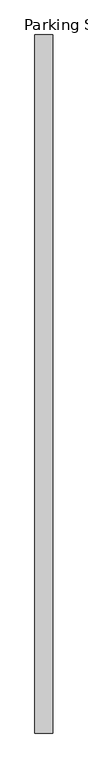
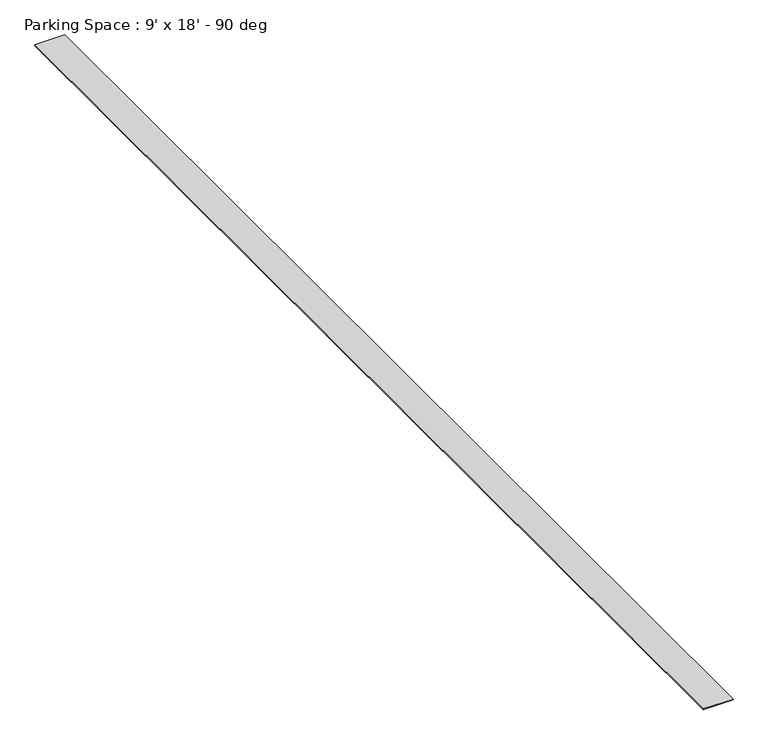
"""IFC4 building model written with IfcOpenShell, lengths in millimetres: proxy geometry, Parking Space : 9' x 18' - 90 deg."""

from ifc_helpers import new_model, si_unit, origin, origin_with_axes, place, context, project, spatial, polyline, outline, extrude, source, transform, mapped, element, save


def parking_space_9_x_18_90_deg_c935943f(model_context):
    return source(origin(), model_context, "Body", "SweptSolid", [
        extrude(outline(polyline([(-50.8, 0.0), (50.8, 0.0), (50.8, -3962.4), (-50.8, -3962.4), (-50.8, 0.0)])), origin_with_axes(), (0.0, 0.0, 1.0), 3.175),
    ])


if __name__ == "__main__":
    model = new_model("IFC4")
    model_context = context("Model", 3, world=origin())
    ifc_project = project(units=[si_unit("LENGTHUNIT", "METRE", prefix="MILLI")], contexts=[model_context])
    site = spatial("IfcSite", under=ifc_project)
    building = spatial("IfcBuilding", under=site)
    placement = place(None, origin())
    parking_space_9_x_18_90_deg_shape = parking_space_9_x_18_90_deg_c935943f(model_context)
    element("IfcBuildingElementProxy", 1, Name="Parking Space : 9' x 18' - 90 deg", ObjectType="Parking Space : 9' x 18' - 90 deg", at=placement, inside=building, context=model_context, shape_type="MappedRepresentation", body=[
        mapped(parking_space_9_x_18_90_deg_shape, transform((0.0, 0.0, 0.0), x_axis=(1.0, 0.0, 0.0), y_axis=(0.0, 1.0, 0.0), z_axis=(0.0, 0.0, 1.0))),
    ])
    save(model, "model.ifc")

# Revit data of these elements
# Type "Parking Space : 9' x 18' - 90 deg"
#   Angle = 90.00°
#   Parking Length = 18' - 0"
#   Parking Width = 9' - 0"
#   pl = 13' - 0"
#   pw = 7' - 0"
# Element 1 (IfcBuildingElementProxy, "Parking Space : 9' x 18' - 90 deg")
#   Materials on its faces: "Parking Stripe"
# Materials
#   "Parking Stripe": class "Paint", colour RGB 250 250 91, transparency 0
